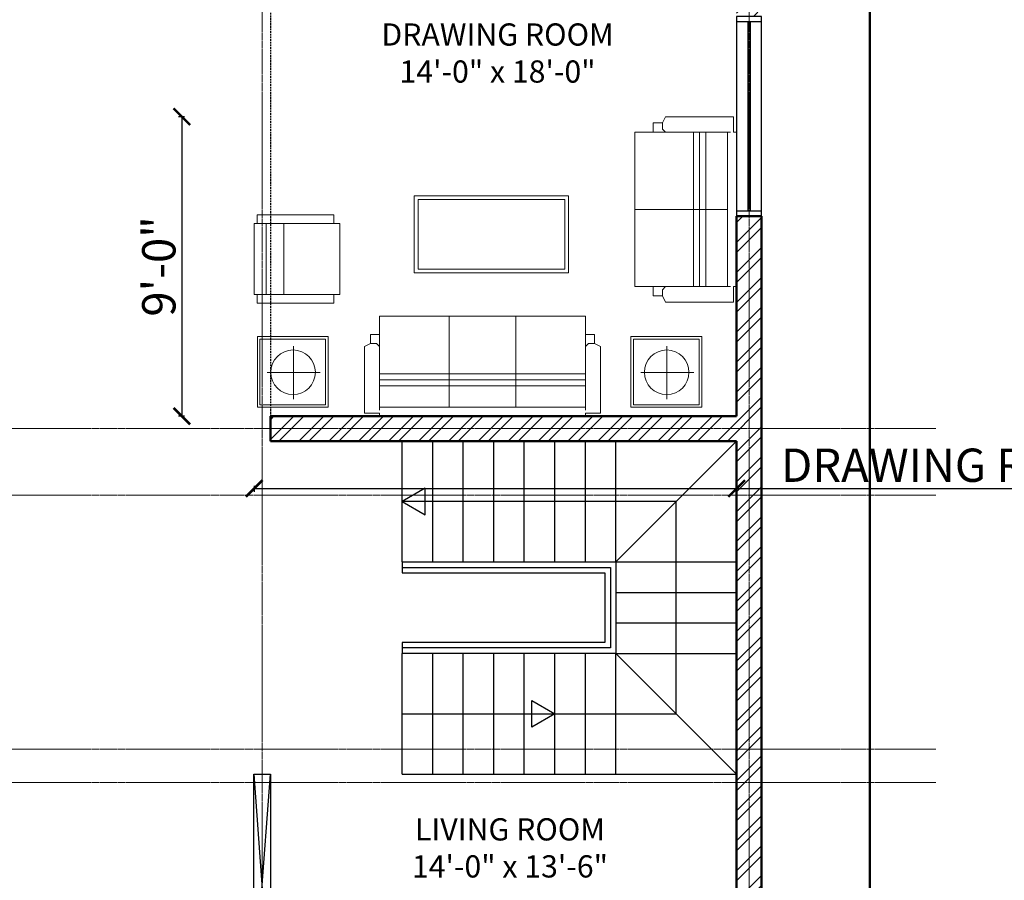
# Model space of a CAD drawing. Units: inches. Extents: x 261 to 2725, y 291 to 1454.
# Tile 12 of 35: x 688 to 1043, y 641 to 951. Entities that reach past the tile are written whole.
import ezdxf

# ---------------------------------------------------------------- set-up
doc = ezdxf.new("R2010")
doc.units = ezdxf.units.IN
doc.linetypes.add('CENTER', pattern=[2, 1.25, -0.25, 0.25, -0.25])
doc.linetypes.add('DASHED', pattern=[19.05, 12.7, -6.35])
for name, color, linetype, lineweight in [('A-ANNO-DIMS', 136, 'Continuous', 18), ('A-AREA-IDEN', 18, 'Continuous', 18), ('A-FLOR-STRS', 42, 'Continuous', 25), ('A-FURN', 30, 'Continuous', 18), ('A-GLAZ', 150, 'Continuous', 25), ('A-GRID', 251, 'CENTER', 13), ('A-ROOF-PRGL', 25, 'Continuous', 25), ('A-WALL', 222, 'Continuous', 50), ('A-WALL-OVHD', 222, 'DASHED', 25), ('A-WALL-PATT', 243, 'Continuous', 13)]:
    doc.layers.add(name, color=color, linetype=linetype, lineweight=lineweight)
doc.styles.get("Standard").update_dxf_attribs({"font": 'arial.ttf'})
doc.dimstyles.new('ISO-25', dxfattribs={"dimtxt": 12, "dimasz": 6, "dimexe": 1.25, "dimexo": 0.625, "dimtad": 1, "dimdec": 0, "dimlunit": 3, "dimtxsty": 'Standard', "dimblk": 'ARCHTICK', "dimcen": 2.5, "dimadec": 0, "dimazin": 0, "dimtfac": 1, "dimtdec": 0, "dimtmove": 0, "dimatfit": 3, "dimfxl": 1, "dimfxlon": 1, "dimarcsym": 0})

# ---------------------------------------------------------------- blocks, each defined once
blk = doc.blocks.new('A$C518662A7')
at = {"linetype": 'ByBlock'}
for p, q in [((855.8, 2302.4), (973.4, 2302.4)), ((855.8, 1784.8), (855.8, 2302.4)), ((973.4, 2326), (2573.4, 2326)), ((973.4, 2302.4), (973.4, 2326)), ((2573.4, 2326), (2573.4, 2302.4)), ((2573.4, 2302.4), (2691.1, 2302.4)), ((2691.1, 2302.4), (2691.1, 1784.8)), ((973.4, 1784.8), (973.4, 2278.9)), ((973.4, 2255.4), (2573.4, 2255.4)), ((1514.6, 1549.5), (1514.6, 2255.4)), ((2032.3, 1549.5), (2032.3, 2255.4)), ((2573.4, 1784.8), (2573.4, 2278.9)), ((2573.4, 2090.7), (973.4, 2090.7)), ((2573.4, 2043.6), (973.4, 2043.6)), ((2573.4, 1996.5), (973.4, 1996.5)), ((902.9, 1761.3), (855.8, 1784.8)), ((902.9, 1761.3), (949.9, 1761.3)), ((902.9, 1690.7), (902.9, 1761.3)), ((949.9, 1761.3), (973.4, 1784.8)), ((973.4, 1690.7), (973.4, 1784.8)), ((2573.4, 1690.7), (2573.4, 1784.8)), ((2597, 1761.3), (2573.4, 1784.8)), ((2644, 1761.3), (2597, 1761.3)), ((2691.1, 1784.8), (2644, 1761.3)), ((2644, 1761.3), (2644, 1690.7)), ((973.4, 1690.7), (902.9, 1690.7)), ((973.4, 1549.5), (973.4, 1690.7)), ((2644, 1690.7), (2573.4, 1690.7)), ((2573.4, 1690.7), (2573.4, 1549.5)), ((2573.4, 1549.5), (973.4, 1549.5)), ((0, 1380.2), (0, 830.2)), ((664.6, 1380.2), (0, 1380.2)), ((22.9, 1448.9), (22.9, 1380.2)), ((618.7, 1448.9), (22.9, 1448.9)), ((91.7, 1380.2), (91.7, 830.2)), ((229.2, 830.2), (229.2, 1380.2)), ((618.7, 1380.2), (618.7, 1448.9)), ((664.6, 830.2), (664.6, 1380.2)), ((3101, 1320), (3101, 1392)), ((3101, 1392), (3173, 1392)), ((3173, 1392), (3197, 1440)), ((3173, 1392), (3173, 1344)), ((3197, 1440), (3725, 1440)), ((3725, 1440), (3725, 1320)), ((2957, 1320), (3101, 1320)), ((2957, 120), (2957, 1320)), ((3101, 1320), (3197, 1320)), ((3173, 1344), (3197, 1320)), ((3197, 1320), (3701, 1320)), ((3413, 120), (3413, 1320)), ((3461, 120), (3461, 1320)), ((3509, 120), (3509, 1320)), ((3677, 1320), (3677, 120)), ((3725, 1320), (3749, 1320)), ((3749, 1320), (3749, 120)), ((0, 830.2), (664.6, 830.2)), ((22.9, 830.2), (22.9, 761.4)), ((618.7, 761.4), (618.7, 830.2)), ((22.9, 761.4), (618.7, 761.4)), ((2957, 720), (3677, 720)), ((3101, 120), (2957, 120)), ((3101, 120), (3197, 120)), ((3101, 48), (3101, 120)), ((3173, 96), (3197, 120)), ((3173, 48), (3173, 96)), ((3197, 120), (3701, 120)), ((3749, 120), (3725, 120)), ((3725, 120), (3725, 0)), ((3173, 48), (3101, 48)), ((3197, 0), (3173, 48)), ((3725, 0), (3197, 0))]:
    blk.add_line(p, q, dxfattribs=at)
for p, q in [((24.2, 2257.5), (574.2, 2257.5)), ((24.2, 1707.5), (24.2, 2257.5)), ((44.2, 2237.5), (554.2, 2237.5)), ((44.2, 1727.5), (44.2, 2237.5)), ((554.2, 2237.5), (554.2, 1727.5)), ((574.2, 2257.5), (574.2, 1707.5)), ((2927.5, 2257.5), (3477.5, 2257.5)), ((2927.5, 1707.5), (2927.5, 2257.5)), ((2947.5, 2237.5), (3457.5, 2237.5)), ((2947.5, 1727.5), (2947.5, 2237.5)), ((3457.5, 2237.5), (3457.5, 1727.5)), ((3477.5, 2257.5), (3477.5, 1707.5)), ((304.4, 2193.4), (304.4, 1783.3)), ((3207.6, 2193.4), (3207.6, 1783.3)), ((100.6, 1987.3), (512.6, 1987.3)), ((3003.8, 1987.3), (3415.8, 1987.3)), ((574.2, 1707.5), (24.2, 1707.5)), ((554.2, 1727.5), (44.2, 1727.5)), ((3477.5, 1707.5), (2927.5, 1707.5)), ((3457.5, 1727.5), (2947.5, 1727.5)), ((1243.6, 1213.6), (2443.6, 1213.6)), ((1243.6, 613.6), (1243.6, 1213.6)), ((1273.6, 1183.6), (2413.6, 1183.6)), ((1273.6, 643.6), (1273.6, 1183.6)), ((2413.6, 1183.6), (2413.6, 643.6)), ((2443.6, 1213.6), (2443.6, 613.6)), ((2443.6, 613.6), (1243.6, 613.6)), ((2413.6, 643.6), (1273.6, 643.6))]:
    blk.add_line(p, q)
for centre in [(302.2, 1985.1), (3205.4, 1985.1)]:
    blk.add_circle(centre, 173.1)
blk = doc.blocks.new('WIN-72')
for p, q in [((955.45, 950.47), (946.45, 950.47)), ((950.45, 950.47), (950.45, 882.47)), ((951.45, 882.47), (951.45, 950.47)), ((946.45, 882.47), (955.45, 882.47))]:
    blk.add_line(p, q)
blk.add_lwpolyline([(955.45, 880.47), (955.45, 952.47), (946.45, 952.47), (946.45, 880.47)], close=True)
blk = doc.blocks.new('_ArchTick')
at = {"color": 0, "linetype": 'ByBlock', "const_width": 0.15}
blk.add_lwpolyline([(-0.5, -0.5), (0.5, 0.5)], dxfattribs=at)
blk = doc.blocks.new('*D69')
at = {"layer": 'A-ANNO-DIMS', "color": 0, "lineweight": -2, "ltscale": 0.07, "transparency": 16777216}
for p, q in [((772.63, 783.4), (772.63, 781.15)), ((772.63, 782.4), (946.45, 782.4)), ((946.45, 783.4), (946.45, 781.15)), ((946.45, 782.4), (1224.37, 782.4))]:
    blk.add_line(p, q, dxfattribs=at)
at = {"layer": 'Defpoints', "color": 0, "ltscale": 0.07, "transparency": 16777216}
for p in [(772.63, 808.47), (946.45, 808.47), (946.45, 782.4)]:
    blk.add_point(p, dxfattribs=at)
at = {"layer": 'A-ANNO-DIMS', "color": 0, "lineweight": -2, "ltscale": 0.07, "transparency": 16777216, "xscale": 6, "yscale": 6, "zscale": 6, "rotation": 180}
blk.add_blockref('_ArchTick', (772.63, 782.4), dxfattribs=at)
at = {"layer": 'A-ANNO-DIMS', "color": 0, "lineweight": -2, "ltscale": 0.07, "transparency": 16777216, "xscale": 6, "yscale": 6, "zscale": 6}
blk.add_blockref('_ArchTick', (946.45, 782.4), dxfattribs=at)
at = {"layer": 'A-ANNO-DIMS', "color": 0, "ltscale": 0.07, "transparency": 16777216, "insert": (1088.41, 789.23), "char_height": 12, "attachment_point": 5}
blk.add_mtext('DRAWING ROOM SOFA SET 14\'-6"', dxfattribs=at)
blk = doc.blocks.new('*D70')
at = {"layer": 'A-ANNO-DIMS', "color": 0, "lineweight": -2, "ltscale": 0.07, "transparency": 16777216}
for p, q in [((747.56, 916.31), (745.31, 916.31)), ((746.56, 916.31), (746.56, 808.47)), ((747.56, 808.47), (745.31, 808.47))]:
    blk.add_line(p, q, dxfattribs=at)
at = {"layer": 'Defpoints', "color": 0, "ltscale": 0.07, "transparency": 16777216}
for p in [(772.63, 916.31), (746.56, 808.47), (772.63, 808.47)]:
    blk.add_point(p, dxfattribs=at)
at = {"layer": 'A-ANNO-DIMS', "color": 0, "lineweight": -2, "ltscale": 0.07, "transparency": 16777216, "xscale": 6, "yscale": 6, "zscale": 6}
for p, rotation in [((746.56, 916.31), 90), ((746.56, 808.47), 270)]:
    blk.add_blockref('_ArchTick', p, dxfattribs=dict(at, rotation=rotation))
at = {"layer": 'A-ANNO-DIMS', "color": 0, "ltscale": 0.07, "transparency": 16777216, "insert": (739.81, 862.39), "char_height": 12, "attachment_point": 5, "rotation": 90}
blk.add_mtext('9\'-0"', dxfattribs=at)
blk = doc.blocks.new('*D82')
at = {"layer": 'A-ANNO-DIMS', "color": 0, "lineweight": -2, "ltscale": 0.07, "transparency": 16777216}
for p, q in [((2600.96, 679.47), (2603.21, 679.47)), ((2601.96, 517.47), (2601.96, 679.47)), ((2600.96, 517.47), (2603.21, 517.47))]:
    blk.add_line(p, q, dxfattribs=at)
at = {"layer": 'Defpoints', "color": 0, "ltscale": 0.07, "transparency": 16777216}
for p in [(946.45, 679.47), (2601.96, 679.47), (946.45, 517.47)]:
    blk.add_point(p, dxfattribs=at)
at = {"layer": 'A-ANNO-DIMS', "color": 0, "lineweight": -2, "ltscale": 0.07, "transparency": 16777216, "xscale": 6, "yscale": 6, "zscale": 6}
for p, rotation in [((2601.96, 679.47), 90), ((2601.96, 517.47), 270)]:
    blk.add_blockref('_ArchTick', p, dxfattribs=dict(at, rotation=rotation))
at = {"layer": 'A-ANNO-DIMS', "color": 0, "ltscale": 0.07, "transparency": 16777216, "insert": (2595.2, 598.47), "char_height": 12, "attachment_point": 5, "rotation": 90}
blk.add_mtext('13\'-6"', dxfattribs=at)
blk = doc.blocks.new('*D83')
at = {"layer": 'A-ANNO-DIMS', "color": 0, "lineweight": -2, "ltscale": 0.07, "transparency": 16777216}
for p, q in [((2600.96, 799.47), (2603.21, 799.47)), ((2601.96, 679.47), (2601.96, 799.47)), ((2600.96, 679.47), (2603.21, 679.47))]:
    blk.add_line(p, q, dxfattribs=at)
at = {"layer": 'Defpoints', "color": 0, "ltscale": 0.07, "transparency": 16777216}
for p in [(946.45, 799.47), (2601.96, 799.47), (946.45, 679.47)]:
    blk.add_point(p, dxfattribs=at)
at = {"layer": 'A-ANNO-DIMS', "color": 0, "lineweight": -2, "ltscale": 0.07, "transparency": 16777216, "xscale": 6, "yscale": 6, "zscale": 6}
for p, rotation in [((2601.96, 799.47), 90), ((2601.96, 679.47), 270)]:
    blk.add_blockref('_ArchTick', p, dxfattribs=dict(at, rotation=rotation))
at = {"layer": 'A-ANNO-DIMS', "color": 0, "ltscale": 0.07, "transparency": 16777216, "insert": (2595.21, 739.47), "char_height": 12, "attachment_point": 5, "rotation": 90}
blk.add_mtext('10\'-0"', dxfattribs=at)
blk = doc.blocks.new('*D84')
at = {"layer": 'A-ANNO-DIMS', "color": 0, "lineweight": -2, "ltscale": 0.07, "transparency": 16777216}
for p, q in [((2600.96, 1024.47), (2603.21, 1024.47)), ((2601.96, 799.47), (2601.96, 1024.47)), ((2600.96, 799.47), (2603.21, 799.47))]:
    blk.add_line(p, q, dxfattribs=at)
at = {"layer": 'Defpoints', "color": 0, "ltscale": 0.07, "transparency": 16777216}
for p in [(946.45, 1024.47), (2601.96, 1024.47), (946.45, 799.47)]:
    blk.add_point(p, dxfattribs=at)
at = {"layer": 'A-ANNO-DIMS', "color": 0, "lineweight": -2, "ltscale": 0.07, "transparency": 16777216, "xscale": 6, "yscale": 6, "zscale": 6}
for p, rotation in [((2601.96, 1024.47), 90), ((2601.96, 799.47), 270)]:
    blk.add_blockref('_ArchTick', p, dxfattribs=dict(at, rotation=rotation))
at = {"layer": 'A-ANNO-DIMS', "color": 0, "ltscale": 0.07, "transparency": 16777216, "insert": (2595.21, 911.97), "char_height": 12, "attachment_point": 5, "rotation": 90}
blk.add_mtext('18\'-9"', dxfattribs=at)
blk = doc.blocks.new('*D86')
at = {"layer": 'A-ANNO-DIMS', "color": 0, "lineweight": -2, "ltscale": 0.07, "transparency": 16777216}
for p, q in [((676.45, 1437.76), (676.45, 1440.01)), ((676.45, 1438.76), (772.45, 1438.76)), ((772.45, 1437.76), (772.45, 1440.01))]:
    blk.add_line(p, q, dxfattribs=at)
at = {"layer": 'Defpoints', "color": 0, "ltscale": 0.07, "transparency": 16777216}
for p in [(772.45, 1438.76), (676.45, 517.47), (772.45, 517.47)]:
    blk.add_point(p, dxfattribs=at)
at = {"layer": 'A-ANNO-DIMS', "color": 0, "lineweight": -2, "ltscale": 0.07, "transparency": 16777216, "xscale": 6, "yscale": 6, "zscale": 6, "rotation": 180}
blk.add_blockref('_ArchTick', (676.45, 1438.76), dxfattribs=at)
at = {"layer": 'A-ANNO-DIMS', "color": 0, "lineweight": -2, "ltscale": 0.07, "transparency": 16777216, "xscale": 6, "yscale": 6, "zscale": 6}
blk.add_blockref('_ArchTick', (772.45, 1438.76), dxfattribs=at)
at = {"layer": 'A-ANNO-DIMS', "color": 0, "ltscale": 0.07, "transparency": 16777216, "insert": (724.45, 1445.51), "char_height": 12, "attachment_point": 5}
blk.add_mtext('8\'-0"', dxfattribs=at)
blk = doc.blocks.new('*D99')
at = {"layer": 'A-ANNO-DIMS', "color": 0, "lineweight": -2, "ltscale": 0.07, "transparency": 16777216}
for p, q in [((825.95, 305.22), (825.95, 302.97)), ((836.95, 305.22), (836.95, 302.97)), ((825.95, 304.22), (836.95, 304.22)), ((836.95, 304.22), (885.42, 304.22))]:
    blk.add_line(p, q, dxfattribs=at)
at = {"layer": 'Defpoints', "color": 0, "ltscale": 0.07, "transparency": 16777216}
for p in [(825.95, 679.47), (836.95, 679.47), (836.95, 304.22)]:
    blk.add_point(p, dxfattribs=at)
at = {"layer": 'A-ANNO-DIMS', "color": 0, "lineweight": -2, "ltscale": 0.07, "transparency": 16777216, "xscale": 6, "yscale": 6, "zscale": 6, "rotation": 180}
blk.add_blockref('_ArchTick', (825.95, 304.22), dxfattribs=at)
at = {"layer": 'A-ANNO-DIMS', "color": 0, "lineweight": -2, "ltscale": 0.07, "transparency": 16777216, "xscale": 6, "yscale": 6, "zscale": 6}
blk.add_blockref('_ArchTick', (836.95, 304.22), dxfattribs=at)
at = {"layer": 'A-ANNO-DIMS', "color": 0, "ltscale": 0.07, "transparency": 16777216, "insert": (864.19, 310.97), "char_height": 12, "attachment_point": 5}
blk.add_mtext('0\'-11"', dxfattribs=at)
blk = doc.blocks.new('*D100')
at = {"layer": 'A-ANNO-DIMS', "color": 0, "lineweight": -2, "ltscale": 0.07, "transparency": 16777216}
for p, q in [((287.06, 799.47), (284.81, 799.47)), ((286.06, 799.47), (286.06, 755.97)), ((287.06, 755.97), (284.81, 755.97)), ((286.06, 755.97), (286.06, 688.87))]:
    blk.add_line(p, q, dxfattribs=at)
at = {"layer": 'Defpoints', "color": 0, "ltscale": 0.07, "transparency": 16777216}
for p in [(825.95, 799.47), (286.06, 755.97), (825.95, 755.97)]:
    blk.add_point(p, dxfattribs=at)
at = {"layer": 'A-ANNO-DIMS', "color": 0, "lineweight": -2, "ltscale": 0.07, "transparency": 16777216, "xscale": 6, "yscale": 6, "zscale": 6}
for p, rotation in [((286.06, 799.47), 90), ((286.06, 755.97), 270)]:
    blk.add_blockref('_ArchTick', p, dxfattribs=dict(at, rotation=rotation))
at = {"layer": 'A-ANNO-DIMS', "color": 0, "ltscale": 0.07, "transparency": 16777216, "insert": (279.22, 719.42), "char_height": 12, "attachment_point": 5, "rotation": 90}
blk.add_mtext('3\'-7 1/2"', dxfattribs=at)
blk = doc.blocks.new('*D101')
at = {"layer": 'A-ANNO-DIMS', "color": 0, "lineweight": -2, "ltscale": 0.07, "transparency": 16777216}
for p, q in [((902.95, 305.22), (902.95, 302.97)), ((946.45, 305.22), (946.45, 302.97)), ((902.95, 304.22), (946.45, 304.22)), ((946.45, 304.22), (1013.55, 304.22))]:
    blk.add_line(p, q, dxfattribs=at)
at = {"layer": 'Defpoints', "color": 0, "ltscale": 0.07, "transparency": 16777216}
for p in [(902.95, 679.47), (946.45, 679.47), (946.45, 304.22)]:
    blk.add_point(p, dxfattribs=at)
at = {"layer": 'A-ANNO-DIMS', "color": 0, "lineweight": -2, "ltscale": 0.07, "transparency": 16777216, "xscale": 6, "yscale": 6, "zscale": 6, "rotation": 180}
blk.add_blockref('_ArchTick', (902.95, 304.22), dxfattribs=at)
at = {"layer": 'A-ANNO-DIMS', "color": 0, "lineweight": -2, "ltscale": 0.07, "transparency": 16777216, "xscale": 6, "yscale": 6, "zscale": 6}
blk.add_blockref('_ArchTick', (946.45, 304.22), dxfattribs=at)
at = {"layer": 'A-ANNO-DIMS', "color": 0, "ltscale": 0.07, "transparency": 16777216, "insert": (983, 311.05), "char_height": 12, "attachment_point": 5}
blk.add_mtext('3\'-7 1/2"', dxfattribs=at)
blk = doc.blocks.new('*D103')
at = {"layer": 'A-ANNO-DIMS', "color": 0, "lineweight": -2, "ltscale": 0.07, "transparency": 16777216}
for p, q in [((287.06, 1231.47), (284.81, 1231.47)), ((286.06, 439.47), (286.06, 1231.47)), ((287.06, 439.47), (284.81, 439.47))]:
    blk.add_line(p, q, dxfattribs=at)
at = {"layer": 'Defpoints', "color": 0, "ltscale": 0.07, "transparency": 16777216}
for p in [(286.06, 1231.47), (1243.08, 1231.47), (1243.08, 439.47)]:
    blk.add_point(p, dxfattribs=at)
at = {"layer": 'A-ANNO-DIMS', "color": 0, "lineweight": -2, "ltscale": 0.07, "transparency": 16777216, "xscale": 6, "yscale": 6, "zscale": 6}
for p, rotation in [((286.06, 1231.47), 90), ((286.06, 439.47), 270)]:
    blk.add_blockref('_ArchTick', p, dxfattribs=dict(at, rotation=rotation))
at = {"layer": 'A-ANNO-DIMS', "color": 0, "ltscale": 0.07, "transparency": 16777216, "insert": (279.3, 835.47), "char_height": 12, "attachment_point": 5, "rotation": 90}
blk.add_mtext('66\'-0"', dxfattribs=at)
blk = doc.blocks.new('*D107')
at = {"layer": 'A-ANNO-DIMS', "color": 0, "lineweight": -2, "ltscale": 0.07, "transparency": 16777216}
for p, q in [((287.06, 673.47), (284.81, 673.47)), ((286.06, 496.47), (286.06, 673.47)), ((287.06, 496.47), (284.81, 496.47))]:
    blk.add_line(p, q, dxfattribs=at)
at = {"layer": 'Defpoints', "color": 0, "ltscale": 0.07, "transparency": 16777216}
for p in [(286.06, 673.47), (1252.08, 673.47), (1252.08, 496.47)]:
    blk.add_point(p, dxfattribs=at)
at = {"layer": 'A-ANNO-DIMS', "color": 0, "lineweight": -2, "ltscale": 0.07, "transparency": 16777216, "xscale": 6, "yscale": 6, "zscale": 6}
for p, rotation in [((286.06, 673.47), 90), ((286.06, 496.47), 270)]:
    blk.add_blockref('_ArchTick', p, dxfattribs=dict(at, rotation=rotation))
at = {"layer": 'A-ANNO-DIMS', "color": 0, "ltscale": 0.07, "transparency": 16777216, "insert": (279.3, 584.97), "char_height": 12, "attachment_point": 5, "rotation": 90}
blk.add_mtext('14\'-9"', dxfattribs=at)
blk = doc.blocks.new('*D108')
at = {"layer": 'A-ANNO-DIMS', "color": 0, "lineweight": -2, "ltscale": 0.07, "transparency": 16777216}
for p, q in [((287.06, 799.47), (284.81, 799.47)), ((286.06, 673.47), (286.06, 799.47)), ((287.06, 673.47), (284.81, 673.47))]:
    blk.add_line(p, q, dxfattribs=at)
at = {"layer": 'Defpoints', "color": 0, "ltscale": 0.07, "transparency": 16777216}
for p in [(286.06, 799.47), (1252.08, 799.47), (1252.08, 673.47)]:
    blk.add_point(p, dxfattribs=at)
at = {"layer": 'A-ANNO-DIMS', "color": 0, "lineweight": -2, "ltscale": 0.07, "transparency": 16777216, "xscale": 6, "yscale": 6, "zscale": 6}
for p, rotation in [((286.06, 799.47), 90), ((286.06, 673.47), 270)]:
    blk.add_blockref('_ArchTick', p, dxfattribs=dict(at, rotation=rotation))
at = {"layer": 'A-ANNO-DIMS', "color": 0, "ltscale": 0.07, "transparency": 16777216, "insert": (279.3, 736.47), "char_height": 12, "attachment_point": 5, "rotation": 90}
blk.add_mtext('10\'-6"', dxfattribs=at)
blk = doc.blocks.new('*D109')
at = {"layer": 'A-ANNO-DIMS', "color": 0, "lineweight": -2, "ltscale": 0.07, "transparency": 16777216}
for p, q in [((287.06, 964.47), (284.81, 964.47)), ((286.06, 799.47), (286.06, 964.47)), ((287.06, 799.47), (284.81, 799.47))]:
    blk.add_line(p, q, dxfattribs=at)
at = {"layer": 'Defpoints', "color": 0, "ltscale": 0.07, "transparency": 16777216}
for p in [(286.06, 964.47), (1252.08, 964.47), (1252.08, 799.47)]:
    blk.add_point(p, dxfattribs=at)
at = {"layer": 'A-ANNO-DIMS', "color": 0, "lineweight": -2, "ltscale": 0.07, "transparency": 16777216, "xscale": 6, "yscale": 6, "zscale": 6}
for p, rotation in [((286.06, 964.47), 90), ((286.06, 799.47), 270)]:
    blk.add_blockref('_ArchTick', p, dxfattribs=dict(at, rotation=rotation))
at = {"layer": 'A-ANNO-DIMS', "color": 0, "ltscale": 0.07, "transparency": 16777216, "insert": (279.3, 881.97), "char_height": 12, "attachment_point": 5, "rotation": 90}
blk.add_mtext('13\'-9"', dxfattribs=at)
blk = doc.blocks.new('*D123')
at = {"layer": 'A-ANNO-DIMS', "color": 0, "lineweight": -2, "ltscale": 0.07, "transparency": 16777216}
for p, q in [((287.06, 1054.85), (284.81, 1054.85)), ((286.06, 439.47), (286.06, 1054.85)), ((287.06, 439.47), (284.81, 439.47))]:
    blk.add_line(p, q, dxfattribs=at)
at = {"layer": 'Defpoints', "color": 0, "ltscale": 0.07, "transparency": 16777216}
for p in [(286.06, 1054.85), (2007.71, 1054.85), (2007.71, 439.47)]:
    blk.add_point(p, dxfattribs=at)
at = {"layer": 'A-ANNO-DIMS', "color": 0, "lineweight": -2, "ltscale": 0.07, "transparency": 16777216, "xscale": 6, "yscale": 6, "zscale": 6}
for p, rotation in [((286.06, 1054.85), 90), ((286.06, 439.47), 270)]:
    blk.add_blockref('_ArchTick', p, dxfattribs=dict(at, rotation=rotation))
at = {"layer": 'A-ANNO-DIMS', "color": 0, "ltscale": 0.07, "transparency": 16777216, "insert": (279.22, 747.16), "char_height": 12, "attachment_point": 5, "rotation": 90}
blk.add_mtext('51\'-3 1/2"', dxfattribs=at)

msp = doc.modelspace()

# ---------------------------------------------------------------- hatches: boundary and pattern name
at = {"layer": 'A-WALL-PATT'}
h = msp.add_hatch(dxfattribs=at)
h.set_pattern_fill('ANSI32', color=256, scale=0.8)
h.paths.add_polyline_path([(478.45, 685.47), (580.45, 685.47), (580.45, 691.47), (577.45, 691.47), (577.45, 694.47), (571.45, 694.47), (571.45, 691.47), (478.45, 691.47), (478.45, 721.47), (469.45, 721.47), (469.45, 508.47), (538.45, 508.47), (538.45, 517.47), (478.45, 517.47)])
h.paths.add_polyline_path([(694.45, 517.47), (676.45, 517.47), (676.45, 646.47), (670.45, 646.47), (670.45, 517.47), (610.45, 517.47), (610.45, 508.47), (694.45, 508.47)])
h.paths.add_polyline_path([(676.45, 784.47), (478.45, 784.47), (478.45, 844.47), (469.45, 844.47), (469.45, 745.47), (478.45, 745.47), (478.45, 775.47), (571.45, 775.47), (571.45, 724.47), (577.45, 724.47), (577.45, 775.47), (670.45, 775.47), (670.45, 691.47), (610.45, 691.47), (610.45, 685.47), (670.45, 685.47), (670.45, 682.47), (676.45, 682.47)])
h.paths.add_polyline_path([(955.45, 880.47), (946.45, 880.47), (946.45, 808.47), (778.45, 808.47), (778.45, 799.47), (946.45, 799.47), (946.45, 517.47), (898.45, 517.47), (898.45, 508.47), (955.45, 508.47)])
h.paths.add_polyline_path([(778.45, 598.47), (772.45, 598.47), (772.45, 517.47), (754.45, 517.47), (754.45, 508.47), (826.45, 508.47), (826.45, 517.47), (778.45, 517.47)])
h.paths.add_polyline_path([(955.45, 1090.47), (946.45, 1090.47), (946.45, 1030.47), (817.45, 1030.47), (817.45, 1024.47), (946.45, 1024.47), (946.45, 952.47), (955.45, 952.47)])
h.paths.add_polyline_path([(955.45, 1231.47), (730.45, 1231.47), (730.45, 1222.47), (772.45, 1222.47), (772.45, 1096.47), (766.45, 1096.47), (766.45, 1090.47), (772.45, 1090.47), (772.45, 1006.47), (712.45, 1006.47), (712.45, 1000.47), (778.45, 1000.47), (778.45, 1024.47), (781.45, 1024.47), (781.45, 1030.47), (778.45, 1030.47), (778.45, 1222.47), (946.45, 1222.47), (946.45, 1162.47), (955.45, 1162.47)])
h.paths.add_polyline_path([(694.45, 1231.47), (619.45, 1231.47), (619.45, 1222.47), (646.45, 1222.47), (646.45, 1039.47), (652.45, 1039.47), (652.45, 1090.47), (736.45, 1090.47), (736.45, 1096.47), (652.45, 1096.47), (652.45, 1222.47), (694.45, 1222.47)])
h.paths.add_polyline_path([(571.45, 1231.47), (469.45, 1231.47), (469.45, 1099.47), (478.45, 1099.47), (478.45, 1144.47), (544.45, 1144.47), (544.45, 1153.47), (538.45, 1153.47), (538.45, 1150.47), (478.45, 1150.47), (478.45, 1222.47), (538.45, 1222.47), (538.45, 1183.47), (544.45, 1183.47), (544.45, 1222.47), (571.45, 1222.47)])
h.paths.add_polyline_path([(538.45, 1006.47), (478.45, 1006.47), (478.45, 1051.47), (469.45, 1051.47), (469.45, 940.47), (478.45, 940.47), (478.45, 1000.47), (538.45, 1000.47)])
h.paths.add_polyline_path([(652.45, 1006.47), (652.45, 1009.47), (646.45, 1009.47), (646.45, 1006.47), (586.45, 1006.47), (586.45, 1000.47), (652.45, 1000.47)])
h.paths.add_polyline_path([(1288.08, 973.47), (1243.08, 973.47), (1243.08, 920.97), (1252.08, 920.97), (1252.08, 964.47), (1288.08, 964.47)], flags=17)
h.paths.add_polyline_path([(1402.08, 805.47), (1252.08, 805.47), (1252.08, 848.97), (1243.08, 848.97), (1243.08, 757.47), (1252.08, 757.47), (1252.08, 799.47), (1294.08, 799.47), (1372.08, 799.47), (1372.08, 779.47), (1372.08, 715.47), (1378.08, 715.47), (1378.08, 799.47), (1402.08, 799.47)])
h.paths.add_polyline_path([(1252.08, 721.47), (1243.08, 721.47), (1243.08, 439.47), (1729.08, 439.47), (1729.08, 709.47), (1720.08, 709.47), (1720.08, 679.47), (1582.08, 679.47), (1582.08, 670.47), (1588.08, 670.47), (1588.08, 673.47), (1720.08, 673.47), (1720.08, 559.47), (1690.08, 559.47), (1690.08, 550.47), (1720.08, 550.47), (1720.08, 448.47), (1252.08, 448.47), (1252.08, 496.47), (1312.08, 496.47), (1312.08, 505.47), (1252.08, 505.47), (1252.08, 673.47), (1405.08, 673.47), (1405.08, 679.47), (1378.08, 679.47), (1378.08, 685.47), (1372.08, 685.47), (1372.08, 679.47), (1252.08, 679.47)])
h.paths.add_polyline_path([(1450.08, 550.47), (1480.08, 550.47), (1480.08, 559.47), (1450.08, 559.47), (1450.08, 679.47), (1441.08, 679.47), (1441.08, 673.47), (1444.08, 673.47), (1444.08, 505.47), (1384.08, 505.47), (1384.08, 496.47), (1450.08, 496.47)], flags=17)
h.paths.add_polyline_path([(1618.08, 559.47), (1588.08, 559.47), (1588.08, 634.47), (1582.08, 634.47), (1582.08, 559.47), (1552.08, 559.47), (1552.08, 550.47), (1618.08, 550.47)], flags=17)
h.paths.add_polyline_path([(1564.08, 964.47), (1630.08, 964.47), (1630.08, 973.47), (1477.08, 973.47), (1477.08, 964.47), (1558.08, 964.47), (1558.08, 926.22), (1558.08, 887.97), (1486.08, 887.97), (1486.08, 881.97), (1558.08, 881.97), (1558.08, 805.47), (1450.08, 805.47), (1450.08, 845.97), (1444.08, 845.97), (1444.08, 805.47), (1438.08, 805.47), (1438.08, 799.47), (1564.08, 799.47)], flags=17)
h.paths.add_polyline_path([(1453.08, 973.47), (1408.08, 973.47), (1408.08, 964.47), (1444.08, 964.47), (1444.08, 881.97), (1450.08, 881.97), (1456.08, 881.97), (1456.08, 887.97), (1450.08, 887.97), (1450.08, 964.47), (1453.08, 964.47)], flags=17)
h.paths.add_polyline_path([(1729.08, 1231.47), (1243.08, 1231.47), (1243.08, 1167.47), (1252.08, 1167.47), (1252.08, 1222.47), (1441.08, 1222.47), (1441.08, 1045.47), (1648.08, 1045.47), (1648.08, 1051.47), (1450.08, 1051.47), (1450.08, 1074.47), (1450.08, 1222.47), (1472.08, 1222.47), (1720.08, 1222.47), (1720.08, 1051.47), (1708.08, 1051.47), (1708.08, 1045.47), (1720.08, 1045.47), (1720.08, 973.47), (1702.08, 973.47), (1702.08, 964.47), (1720.08, 964.47), (1720.08, 769.47), (1729.08, 769.47)])
h.paths.add_polyline_path([(2493.71, 1054.85), (2007.71, 1054.85), (2007.71, 439.47), (2214.67, 439.47), (2214.67, 496.47), (2493.71, 496.47)])
h.paths.add_polyline_path([(2016.71, 1045.85), (2304.71, 1045.85), (2304.71, 841.47), (2310.71, 841.47), (2310.71, 1045.85), (2484.71, 1045.85), (2484.71, 805.47), (2310.71, 805.47), (2310.71, 811.47), (2304.71, 811.47), (2304.71, 799.47), (2484.71, 799.47), (2484.71, 679.47), (2304.71, 679.47), (2304.71, 673.47), (2484.71, 673.47), (2484.71, 505.47), (2208.67, 505.47), (2208.67, 448.47), (2016.71, 448.47), (2016.71, 799.47), (2304.71, 799.47), (2304.71, 805.47), (2016.71, 805.47)], flags=16)

# ---------------------------------------------------------------- linework, layer by layer
at = {"layer": 'A-FLOR-STRS'}
for p, q in [((825.95, 755.97), (825.95, 799.47)), ((825.95, 799.47), (946.45, 799.47)), ((836.95, 755.97), (836.95, 799.47)), ((847.95, 755.97), (847.95, 799.47)), ((858.95, 755.97), (858.95, 799.47)), ((869.95, 755.97), (869.95, 799.47)), ((880.95, 755.97), (880.95, 799.47)), ((891.95, 755.97), (891.95, 799.47)), ((902.95, 755.97), (902.95, 799.47)), ((902.95, 755.97), (946.45, 799.47)), ((946.45, 679.47), (946.45, 799.47)), ((924.7, 777.72), (825.95, 777.72)), ((924.7, 701.22), (924.7, 777.72)), ((825.95, 755.97), (825.95, 751.97)), ((902.95, 755.97), (946.45, 755.97)), ((902.95, 744.97), (946.45, 744.97)), ((902.95, 733.97), (946.45, 733.97)), ((825.95, 726.97), (825.95, 722.97)), ((825.95, 679.47), (825.95, 722.97)), ((836.95, 679.47), (836.95, 722.97)), ((847.95, 679.47), (847.95, 722.97)), ((858.95, 679.47), (858.95, 722.97)), ((869.95, 679.47), (869.95, 722.97)), ((880.95, 679.47), (880.95, 722.97)), ((891.95, 679.47), (891.95, 722.97)), ((902.95, 722.97), (946.45, 722.97)), ((902.95, 679.47), (902.95, 722.97)), ((902.95, 722.97), (946.45, 679.47)), ((825.95, 701.22), (924.7, 701.22)), ((825.95, 679.47), (946.45, 679.47))]:
    msp.add_line(p, q, dxfattribs=at)
for points in [[(825.95, 777.72), (834.2, 772.96), (834.2, 782.48)], [(880.95, 701.22), (872.7, 696.46), (872.7, 705.98)]]:
    msp.add_lwpolyline(points, close=True, dxfattribs=at)
for points in [[(825.95, 755.97), (902.95, 755.97), (902.95, 722.97), (825.95, 722.97)], [(825.95, 753.97), (900.95, 753.97), (900.95, 724.97), (825.95, 724.97)], [(825.95, 751.97), (898.95, 751.97), (898.95, 726.97), (825.95, 726.97)]]:
    msp.add_lwpolyline(points, dxfattribs=at)
at = {"layer": 'A-GRID', "ltscale": 0.5}
for p, q in [((775.45, 1330.47), (775.45, 416.47)), ((950.95, 1330.47), (950.95, 416.47)), ((394.31, 803.97), (1018.31, 803.97)), ((394.31, 779.97), (1018.31, 779.97)), ((394.31, 688.47), (1018.31, 688.47)), ((394.31, 676.47), (1018.31, 676.47))]:
    msp.add_line(p, q, dxfattribs=at)
at = {"layer": 'A-ROOF-PRGL'}
for p, q in [((772.45, 598.47), (778.45, 679.47)), ((772.45, 679.47), (778.45, 598.47))]:
    msp.add_line(p, q, dxfattribs=at)
msp.add_lwpolyline([(772.45, 679.47), (778.45, 679.47), (778.45, 598.47), (772.45, 598.47)], close=True, dxfattribs=at)
at = {"layer": 'A-WALL'}
for p, q in [((994.45, 1270.47), (994.45, 412.47)), ((946.45, 880.47), (955.45, 880.47)), ((946.45, 880.47), (946.45, 808.47)), ((955.45, 880.47), (955.45, 508.47)), ((778.45, 808.47), (946.45, 808.47)), ((778.45, 808.47), (778.45, 799.47)), ((778.45, 799.47), (946.45, 799.47)), ((946.45, 517.47), (946.45, 799.47))]:
    msp.add_line(p, q, dxfattribs=at)
at = {"layer": 'A-WALL-OVHD', "ltscale": 0.05}
msp.add_line((778.45, 1000.47), (778.45, 799.47), dxfattribs=at)

# ---------------------------------------------------------------- block references
at = {"layer": 'A-FURN', "xscale": -0.0463636363636368, "yscale": 0.0463636363636368, "zscale": 0.0463636363636368, "rotation": 180}
msp.add_blockref('A$C518662A7', (772.63, 916.31), dxfattribs=at)
at = {"layer": 'A-GLAZ'}
msp.add_blockref('WIN-72', (0, 0), dxfattribs=at)

# ---------------------------------------------------------------- texts
at = {"layer": 'A-AREA-IDEN', "char_height": 8, "attachment_point": 1}
for s, width, insert in [('\\pxqc;{\\fTimes New Roman|b0|i0|c0|p18;DRAWING ROOM\\P14\'-0" x 18\'-0"}', 104.6719, (807.96, 949.94)), ('\\pxqc;{\\fTimes New Roman|b0|i0|c0|p18;LIVING ROOM\\P14\'-0" x 13\'-6"}', 111.8066, (808.86, 663.61))]:
    msp.add_mtext_dynamic_manual_height_columns(s, width=width, gutter_width=12.5, heights=[0], dxfattribs=dict(at, insert=insert))

# ---------------------------------------------------------------- dimensions: what is measured, and where the dimension line sits
at = {"layer": 'A-ANNO-DIMS', "ltscale": 0.07}
for base, p1, p2, picture, middle in [((772.45, 1438.76), (676.45, 517.47), (772.45, 517.47), '*D86', (724.45, 1445.51)), ((836.95, 304.22), (825.95, 679.47), (836.95, 679.47), '*D99', (864.19, 310.97)), ((946.45, 304.22), (902.95, 679.47), (946.45, 679.47), '*D101', (983, 311.05))]:
    dim = msp.add_linear_dim(base=base, p1=p1, p2=p2, dimstyle='ISO-25', override={"dimdec": 1, "dimlfac": 1, "dimrnd": 0, "dimzin": 1, "dimdsep": 46, "dimlunit": 4, "dimfrac": 2}, dxfattribs=at)
    dim.commit()
    dim.dimension.update_dxf_attribs({"geometry": picture, "text_midpoint": middle})
for base, p1, p2, angle, override, picture, middle in [((286.06, 1231.47), (1243.08, 439.47), (1243.08, 1231.47), 90, {"dimdec": 1, "dimlfac": 1, "dimrnd": 0, "dimzin": 1, "dimdsep": 46, "dimlunit": 4, "dimfrac": 2}, '*D103', (279.3, 835.47)), ((286.06, 1054.85), (2007.71, 439.47), (2007.71, 1054.85), 90, {"dimdec": 1, "dimlfac": 1, "dimrnd": 0, "dimzin": 1, "dimdsep": 46, "dimlunit": 4, "dimfrac": 2}, '*D123', (279.22, 747.16)), ((2601.96, 1024.47), (946.45, 799.47), (946.45, 1024.47), 90, {"dimdec": 1, "dimlfac": 1, "dimrnd": 0, "dimzin": 1, "dimdsep": 46, "dimlunit": 4, "dimfrac": 2}, '*D84', (2595.21, 911.97)), ((286.06, 964.47), (1252.08, 799.47), (1252.08, 964.47), 90, {"dimdec": 1, "dimlfac": 1, "dimrnd": 0, "dimzin": 1, "dimdsep": 46, "dimlunit": 4, "dimfrac": 2}, '*D109', (279.3, 881.97)), ((746.56, 808.47), (772.63, 916.31), (772.63, 808.47), 270, {"dimdec": 1, "dimrnd": 0, "dimzin": 1, "dimlunit": 4, "dimfrac": 2}, '*D70', (739.81, 862.39)), ((286.06, 755.97), (825.95, 799.47), (825.95, 755.97), 90, {"dimdec": 1, "dimlfac": 1, "dimrnd": 0, "dimzin": 1, "dimdsep": 46, "dimlunit": 4, "dimfrac": 2}, '*D100', (279.22, 719.42)), ((286.06, 799.47), (1252.08, 673.47), (1252.08, 799.47), 90, {"dimdec": 1, "dimlfac": 1, "dimrnd": 0, "dimzin": 1, "dimdsep": 46, "dimlunit": 4, "dimfrac": 2}, '*D108', (279.3, 736.47)), ((2601.96, 799.47), (946.45, 679.47), (946.45, 799.47), 90, {"dimdec": 1, "dimlfac": 1, "dimrnd": 0, "dimzin": 1, "dimdsep": 46, "dimlunit": 4, "dimfrac": 2}, '*D83', (2595.21, 739.47)), ((2601.96, 679.47), (946.45, 517.47), (946.45, 679.47), 90, {"dimdec": 1, "dimlfac": 1, "dimrnd": 0, "dimzin": 1, "dimdsep": 46, "dimlunit": 4, "dimfrac": 2}, '*D82', (2595.2, 598.47)), ((286.06, 673.47), (1252.08, 496.47), (1252.08, 673.47), 90, {"dimdec": 1, "dimlfac": 1, "dimrnd": 0, "dimzin": 1, "dimdsep": 46, "dimlunit": 4, "dimfrac": 2}, '*D107', (279.3, 584.97))]:
    dim = msp.add_linear_dim(base=base, p1=p1, p2=p2, angle=angle, dimstyle='ISO-25', override=override, dxfattribs=at)
    dim.commit()
    dim.dimension.update_dxf_attribs({"geometry": picture, "text_midpoint": middle})
dim = msp.add_linear_dim(base=(946.45, 782.4), p1=(772.63, 808.47), p2=(946.45, 808.47), text='DRAWING ROOM SOFA SET <>', dimstyle='ISO-25', override={"dimdec": 1, "dimrnd": 0, "dimzin": 1, "dimlunit": 4, "dimfrac": 2}, dxfattribs=at)
dim.commit()
dim.dimension.update_dxf_attribs({"geometry": '*D69', "text_midpoint": (1088.41, 789.23)})

doc.saveas('drawing.dxf')
